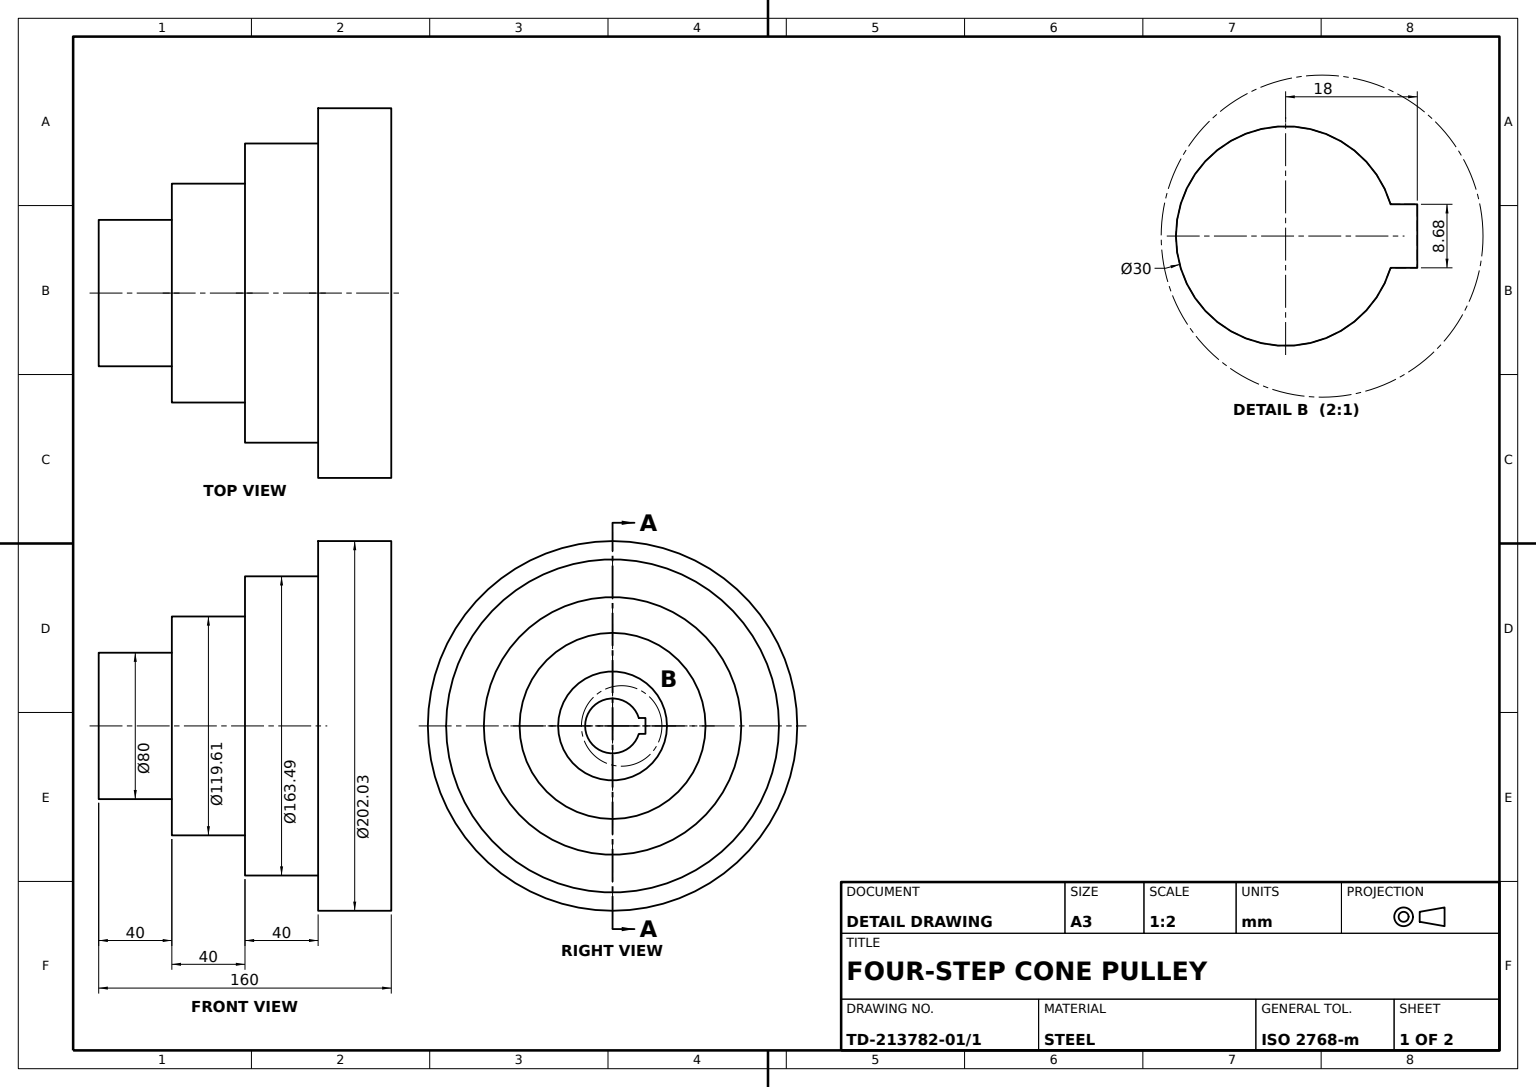
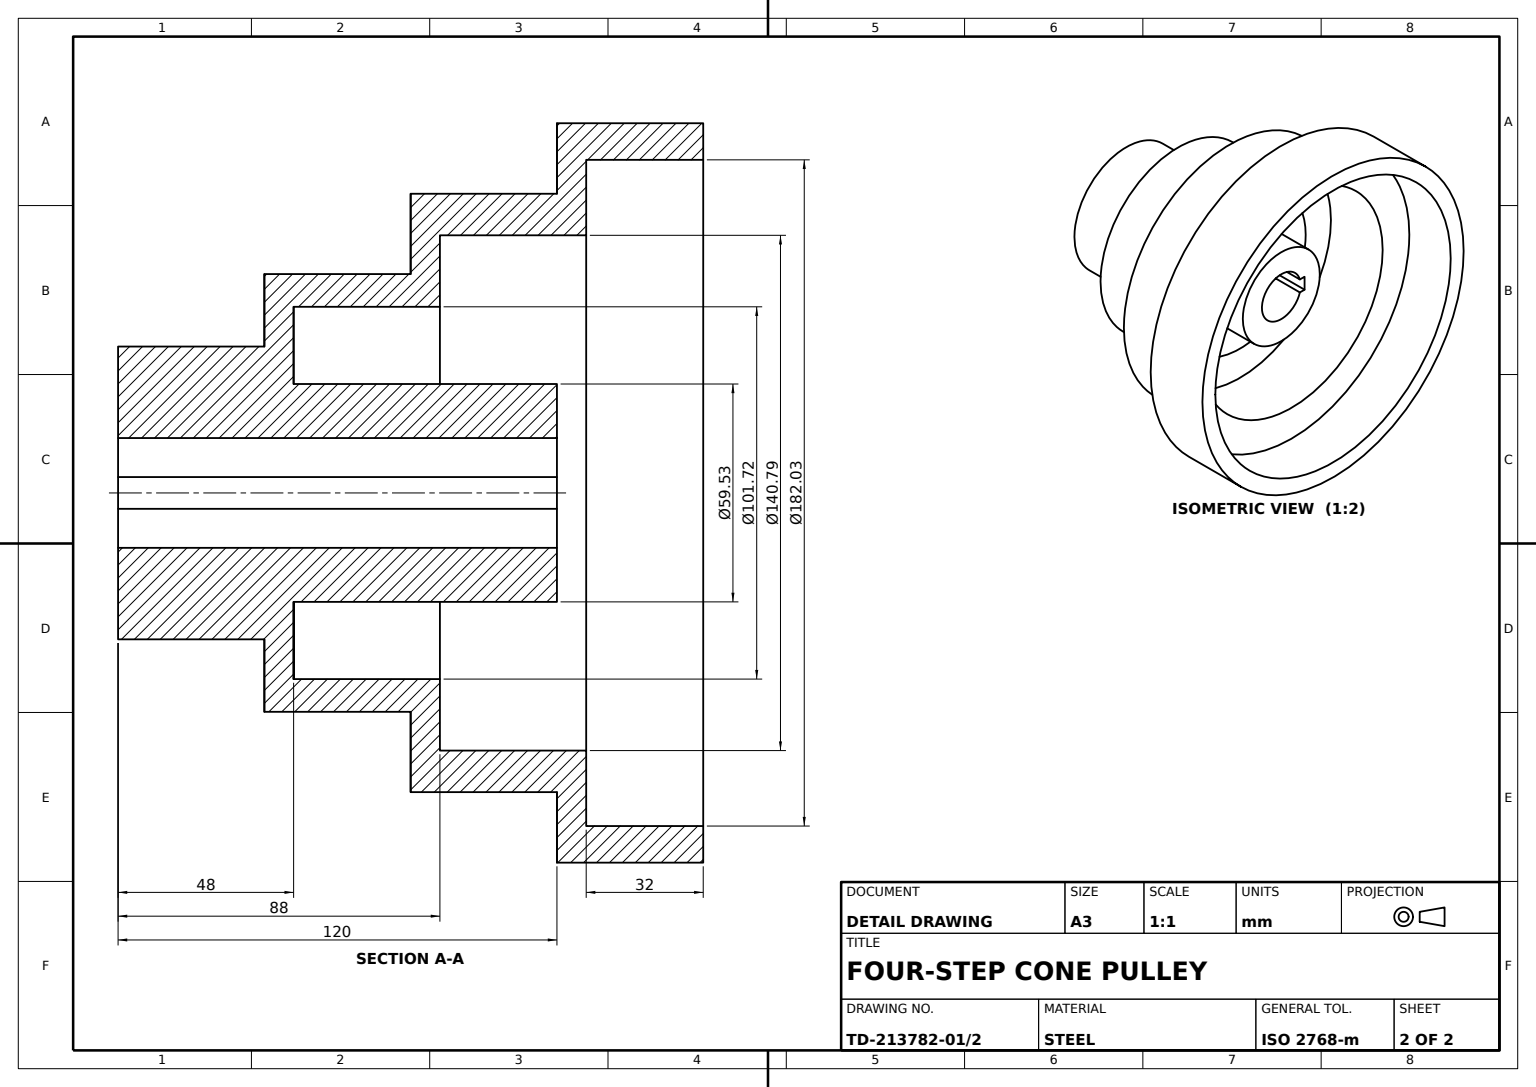
from build123d import *

# Parameters (mm, degrees)
BORE_AND_KEYWAY_PROFILE_W    = 15
BORE_AND_KEYWAY_PROFILE_H    = 8.680150088
SHAFT_BORE_WITH_KEYWAY_DEPTH = 110


with BuildPart() as part:
    # Stepped Pulley Profile → Stepped Pulley Body (revolve)
    with BuildSketch(Plane.XY, mode=Mode.PRIVATE) as stepped_pulley_body_sk:
        Polygon((-55.070008805, 15), (-55.070008805, 40), (-15.070008805, 40), (-15.070008805, 59.802619068), (24.929991195, 59.802619068), (24.929991195, 81.746061819), (64.929991195, 81.746061819), (64.929991195, 101.013474967), (104.929991195, 101.013474967), (104.929991195, 91.013474967), (72.929991195, 91.013474967), (72.929991195, 70.393812799), (32.929991195, 70.393812799), (32.929991195, 50.858796691), (-7.070008805, 50.858796691), (-7.070008805, 29.765145873), (64.929991195, 29.765145873), (64.929991195, 15), align=None)
    revolve(stepped_pulley_body_sk.sketch.rotate(Axis((151.689826596, 0, 0), (-1, 0, 0)), 90), axis=Axis((151.689826596, 0, 0), (-1, 0, 0)))

    # Bore and Keyway Profile → Shaft Bore with Keyway (cut, symmetric)
    with BuildSketch(Plane(origin=(0, 0, 0), x_dir=(0, 0, -1), z_dir=(1, 0, 0))):
        with Locations((10.5, 0)):
            Rectangle(BORE_AND_KEYWAY_PROFILE_W, BORE_AND_KEYWAY_PROFILE_H)
    extrude(amount=SHAFT_BORE_WITH_KEYWAY_DEPTH, both=True, mode=Mode.SUBTRACT)


solid = part.part
